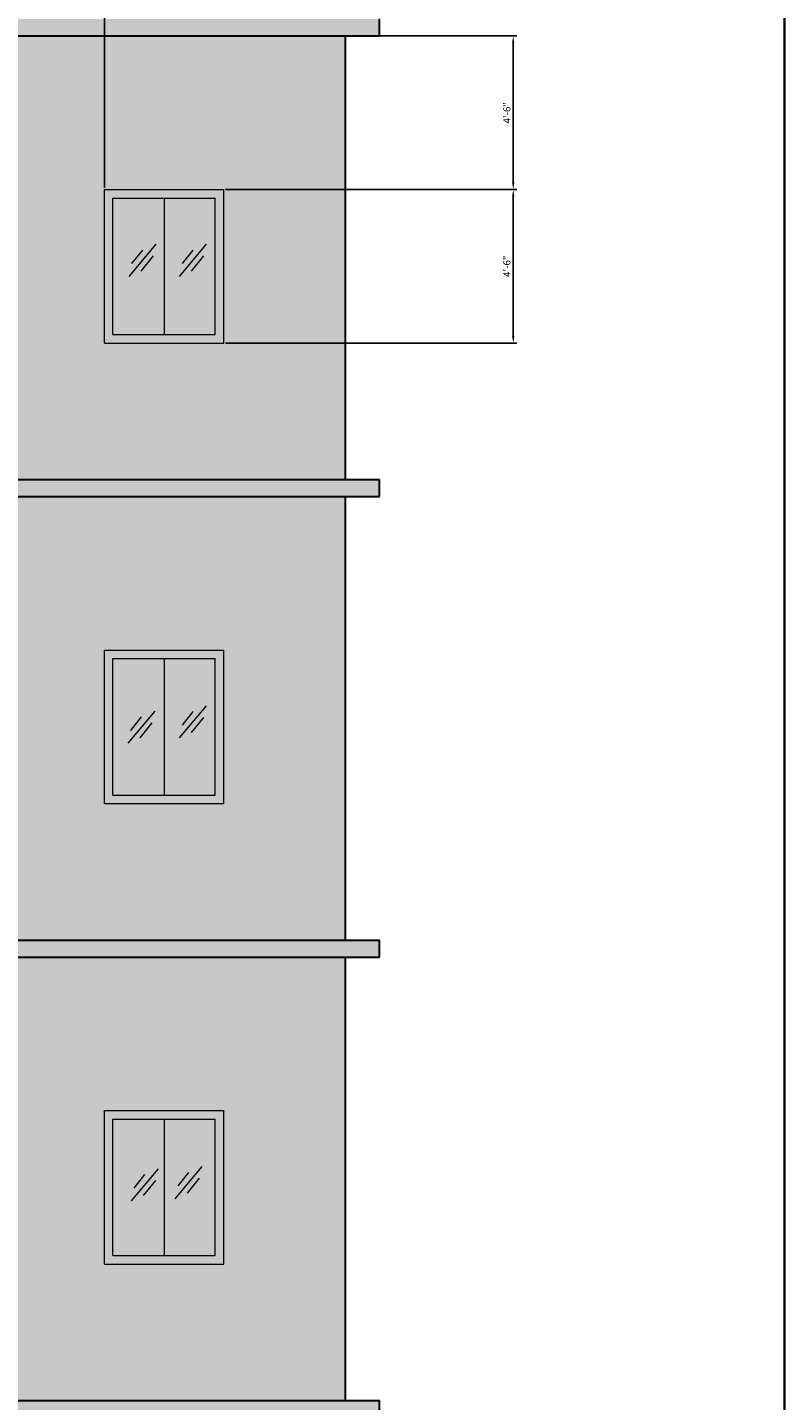
# Model space of a CAD drawing. Units: inches. Extents: x 2391 to 16591, y 7259 to 10239.
# Tile 15 of 27: x 3888 to 4154, y 7746 to 8229. Entities that reach past the tile are written whole.
import ezdxf

# ---------------------------------------------------------------- set-up
doc = ezdxf.new("R2010")
doc.units = ezdxf.units.IN
for name, color, linetype, lineweight in [('A-ANNO-DIMS', 4, 'Continuous', 18), ('A-ANNO-TTLB', 7, 'Continuous', 35), ('A-ELEV', 7, 'Continuous', 30), ('A-ELEV-GLAZ', 4, 'Continuous', 18), ('A-ELEV-GLAZ-PATT', 141, 'Continuous', 13), ('A-ELEV-PATT', 8, 'Continuous', 13), ('A-ELEV-SURF-PATT', 253, 'Continuous', 13)]:
    doc.layers.add(name, color=color, linetype=linetype, lineweight=lineweight)
doc.styles.get("Standard").update_dxf_attribs({"font": 'arial.ttf'})
doc.dimstyles.new('ISO-25', dxfattribs={"dimtxt": 2.5, "dimasz": 2.5, "dimexe": 1.25, "dimexo": 0.625, "dimtad": 1, "dimdec": 0, "dimlunit": 3, "dimtxsty": 'Standard', "dimcen": 2.5, "dimadec": 0, "dimazin": 0, "dimtfac": 1, "dimtdec": 0, "dimtmove": 0, "dimatfit": 3, "dimfxl": 1, "dimarcsym": 0})

# ---------------------------------------------------------------- blocks, each defined once
blk = doc.blocks.new('GLASS-REFLECTION-WINDOW')
for p, q in [((0, 0), (9.5, 11.3)), ((1, 4.52), (4.76, 9.26)), ((4.26, 1.91), (8.52, 7.21))]:
    blk.add_line(p, q)
blk = doc.blocks.new('*D95')
at = {"layer": 'A-ANNO-DIMS', "color": 0, "lineweight": -2, "transparency": 16777216}
for p, q in [((3802.21, 8172.81), (3802.21, 8381.48)), ((3804.71, 8380.23), (3912.46, 8380.23)), ((3914.96, 8172.81), (3914.96, 8381.48))]:
    blk.add_line(p, q, dxfattribs=at)
at = {"layer": 'A-ANNO-DIMS', "color": 0, "transparency": 16777216}
for points in [[(3804.71, 8380.65), (3804.71, 8379.81), (3802.21, 8380.23)], [(3912.46, 8380.65), (3912.46, 8379.81), (3914.96, 8380.23)]]:
    blk.add_solid(points, dxfattribs=at)
at = {"layer": 'Defpoints', "color": 0, "transparency": 16777216}
for p in [(3914.96, 8380.23), (3802.21, 8172.18), (3914.96, 8172.18)]:
    blk.add_point(p, dxfattribs=at)
at = {"layer": 'A-ANNO-DIMS', "color": 0, "transparency": 16777216, "insert": (3858.58, 8382.13), "char_height": 2.5, "attachment_point": 5}
blk.add_mtext('9\'-5"', dxfattribs=at)
blk = doc.blocks.new('*D96')
at = {"layer": 'A-ANNO-DIMS', "color": 0, "lineweight": -2, "transparency": 16777216}
for p, q in [((4000.33, 8226.18), (4060.01, 8226.18)), ((4058.76, 8223.68), (4058.76, 8174.68)), ((3957.58, 8172.18), (4060.01, 8172.18))]:
    blk.add_line(p, q, dxfattribs=at)
at = {"layer": 'A-ANNO-DIMS', "color": 0, "transparency": 16777216}
for points in [[(4058.34, 8223.68), (4059.18, 8223.68), (4058.76, 8226.18)], [(4058.34, 8174.68), (4059.18, 8174.68), (4058.76, 8172.18)]]:
    blk.add_solid(points, dxfattribs=at)
at = {"layer": 'Defpoints', "color": 0, "transparency": 16777216}
for p in [(3999.71, 8226.18), (3956.96, 8172.18), (4058.76, 8172.18)]:
    blk.add_point(p, dxfattribs=at)
at = {"layer": 'A-ANNO-DIMS', "color": 0, "transparency": 16777216, "insert": (4056.86, 8199.18), "char_height": 2.5, "attachment_point": 5, "rotation": 90}
blk.add_mtext('4\'-6"', dxfattribs=at)
blk = doc.blocks.new('*D97')
at = {"layer": 'A-ANNO-DIMS', "color": 0, "lineweight": -2, "transparency": 16777216}
for p, q in [((3957.58, 8172.18), (4060.01, 8172.18)), ((4058.76, 8169.68), (4058.76, 8120.68)), ((3957.58, 8118.18), (4060.01, 8118.18))]:
    blk.add_line(p, q, dxfattribs=at)
at = {"layer": 'A-ANNO-DIMS', "color": 0, "transparency": 16777216}
for points in [[(4058.34, 8169.68), (4059.18, 8169.68), (4058.76, 8172.18)], [(4058.34, 8120.68), (4059.18, 8120.68), (4058.76, 8118.18)]]:
    blk.add_solid(points, dxfattribs=at)
at = {"layer": 'Defpoints', "color": 0, "transparency": 16777216}
for p in [(3956.96, 8172.18), (3956.96, 8118.18), (4058.76, 8118.18)]:
    blk.add_point(p, dxfattribs=at)
at = {"layer": 'A-ANNO-DIMS', "color": 0, "transparency": 16777216, "insert": (4056.86, 8145.18), "char_height": 2.5, "attachment_point": 5, "rotation": 90}
blk.add_mtext('4\'-6"', dxfattribs=at)

msp = doc.modelspace()

# ---------------------------------------------------------------- hatches: boundary and pattern name
at = {"layer": 'A-ELEV-GLAZ-PATT'}
h = msp.add_hatch(color=256, dxfattribs=at)
h.dxf.hatch_style = 1
h.paths.add_polyline_path([(3750.21, 8172.18), (3720.21, 8172.18), (3720.21, 8154.18), (3750.21, 8154.18)])
h.paths.add_polyline_path([(3747.21, 8169.18), (3747.21, 8157.18), (3723.21, 8157.18), (3723.21, 8169.18)], flags=16)
h.paths.add_polyline_path([(3802.21, 8172.18), (3802.21, 8118.18), (3844.21, 8118.18), (3844.21, 8172.18)])
h.paths.add_polyline_path([(3841.21, 8169.18), (3841.21, 8121.18), (3805.21, 8121.18), (3805.21, 8169.18)], flags=16)
h.paths.add_polyline_path([(3956.96, 8172.18), (3914.96, 8172.18), (3914.96, 8118.18), (3956.96, 8118.18)])
h.paths.add_polyline_path([(3953.96, 8169.18), (3953.96, 8121.18), (3917.96, 8121.18), (3917.96, 8169.18)], flags=16)
h.paths.add_polyline_path([(3720.21, 8010.18), (3720.21, 7992.18), (3750.21, 7992.18), (3750.21, 8010.18)])
h.paths.add_polyline_path([(3747.21, 8007.18), (3747.21, 7995.18), (3723.21, 7995.18), (3723.21, 8007.18)], flags=16)
h.paths.add_polyline_path([(3802.21, 8010.18), (3802.21, 7956.18), (3844.21, 7956.18), (3844.21, 8010.18)])
h.paths.add_polyline_path([(3841.21, 8007.18), (3841.21, 7959.18), (3805.21, 7959.18), (3805.21, 8007.18)], flags=16)
h.paths.add_polyline_path([(3914.96, 8010.18), (3914.96, 7956.18), (3956.96, 7956.18), (3956.96, 8010.18)])
h.paths.add_polyline_path([(3917.96, 8007.18), (3953.96, 8007.18), (3953.96, 7959.18), (3917.96, 7959.18)], flags=16)
h.paths.add_polyline_path([(3750.21, 7848.18), (3720.21, 7848.18), (3720.21, 7830.18), (3750.21, 7830.18)])
h.paths.add_polyline_path([(3747.21, 7845.18), (3747.21, 7833.18), (3723.21, 7833.18), (3723.21, 7845.18)], flags=16)
h.paths.add_polyline_path([(3844.21, 7848.18), (3802.21, 7848.18), (3802.21, 7794.18), (3844.21, 7794.18)])
h.paths.add_polyline_path([(3805.21, 7845.18), (3841.21, 7845.18), (3841.21, 7797.18), (3805.21, 7797.18)], flags=16)
h.paths.add_polyline_path([(3914.96, 7848.18), (3914.96, 7794.18), (3956.96, 7794.18), (3956.96, 7848.18)])
h.paths.add_polyline_path([(3917.96, 7845.18), (3953.96, 7845.18), (3953.96, 7797.18), (3917.96, 7797.18)], flags=16)
h = msp.add_hatch(color=256, dxfattribs=at)
h.dxf.hatch_style = 1
h.paths.add_polyline_path([(3735.21, 8169.18), (3723.21, 8169.18), (3723.21, 8157.18), (3735.21, 8157.18)])
h.paths.add_polyline_path([(3747.21, 8169.18), (3735.21, 8169.18), (3735.21, 8157.18), (3747.21, 8157.18)])
h.paths.add_polyline_path([(3823.21, 8169.18), (3805.21, 8169.18), (3805.21, 8121.18), (3823.21, 8121.18)])
h.paths.add_polyline_path([(3841.21, 8169.18), (3823.21, 8169.18), (3823.21, 8121.18), (3841.21, 8121.18)])
h.paths.add_polyline_path([(3935.96, 8169.18), (3917.96, 8169.18), (3917.96, 8121.18), (3935.96, 8121.18)])
h.paths.add_polyline_path([(3953.96, 8169.18), (3935.96, 8169.18), (3935.96, 8121.18), (3953.96, 8121.18)])
h.paths.add_polyline_path([(3735.21, 8007.18), (3723.21, 8007.18), (3723.21, 7995.18), (3735.21, 7995.18)])
h.paths.add_polyline_path([(3747.21, 8007.18), (3735.21, 8007.18), (3735.21, 7995.18), (3747.21, 7995.18)])
h.paths.add_polyline_path([(3823.21, 8007.18), (3805.21, 8007.18), (3805.21, 7959.18), (3823.21, 7959.18)])
h.paths.add_polyline_path([(3841.21, 8007.18), (3823.21, 8007.18), (3823.21, 7959.18), (3841.21, 7959.18)])
h.paths.add_polyline_path([(3935.96, 8007.18), (3917.96, 8007.18), (3917.96, 7959.18), (3935.96, 7959.18)])
h.paths.add_polyline_path([(3953.96, 8007.18), (3935.96, 8007.18), (3935.96, 7959.18), (3953.96, 7959.18)])
h.paths.add_polyline_path([(3735.21, 7845.18), (3723.21, 7845.18), (3723.21, 7833.18), (3735.21, 7833.18)])
h.paths.add_polyline_path([(3747.21, 7845.18), (3735.21, 7845.18), (3735.21, 7833.18), (3747.21, 7833.18)])
h.paths.add_polyline_path([(3823.21, 7845.18), (3805.21, 7845.18), (3805.21, 7797.18), (3823.21, 7797.18)])
h.paths.add_polyline_path([(3841.21, 7845.18), (3823.21, 7845.18), (3823.21, 7797.18), (3841.21, 7797.18)])
h.paths.add_polyline_path([(3935.96, 7845.18), (3917.96, 7845.18), (3917.96, 7797.18), (3935.96, 7797.18)])
h.paths.add_polyline_path([(3953.96, 7845.18), (3935.96, 7845.18), (3935.96, 7797.18), (3953.96, 7797.18)])
at = {"layer": 'A-ELEV-PATT'}
h = msp.add_hatch(dxfattribs=at)
h.set_pattern_fill('BRSTONE', color=256)
h.paths.add_polyline_path([(3999.71, 8226.18), (3881.21, 8226.18), (3881.21, 8070.18), (3999.71, 8070.18)])
h.paths.add_polyline_path([(3956.96, 8118.18), (3914.96, 8118.18), (3914.96, 8172.18), (3956.96, 8172.18)], flags=16)
h.paths.add_polyline_path([(3953.96, 8121.18), (3917.96, 8121.18), (3917.96, 8169.18), (3953.96, 8169.18)], flags=0)
h.paths.add_polyline_path([(3999.71, 8064.18), (3881.21, 8064.18), (3881.21, 7908.18), (3999.71, 7908.18)])
h.paths.add_polyline_path([(3956.96, 7956.18), (3914.96, 7956.18), (3914.96, 8010.18), (3956.96, 8010.18)], flags=16)
h.paths.add_polyline_path([(3953.96, 7959.18), (3917.96, 7959.18), (3917.96, 8007.18), (3953.96, 8007.18)], flags=0)
h.paths.add_polyline_path([(3999.71, 7902.18), (3881.21, 7902.18), (3881.21, 7746.18), (3999.71, 7746.18)])
h.paths.add_polyline_path([(3956.96, 7794.18), (3914.96, 7794.18), (3914.96, 7848.18), (3956.96, 7848.18)], flags=16)
h.paths.add_polyline_path([(3953.96, 7797.18), (3917.96, 7797.18), (3917.96, 7845.18), (3953.96, 7845.18)], flags=0)
h.paths.add_polyline_path([(3999.71, 7740.18), (3567.71, 7740.18), (3567.71, 7697.18), (3760.71, 7697.18), (3760.71, 7706.18), (3755.71, 7706.18), (3755.71, 7711.18), (3774.71, 7711.18), (3774.71, 7706.18), (3769.71, 7706.18), (3769.71, 7677.02), (3772.21, 7677.02), (3772.21, 7679.02), (3774.71, 7679.02), (3774.71, 7704.18), (3843.71, 7704.18), (3843.71, 7589.18), (3774.71, 7589.18), (3774.71, 7584.18), (3913.71, 7584.18), (3913.71, 7589.18), (3844.71, 7589.18), (3844.71, 7704.18), (3913.71, 7704.18), (3913.71, 7679.02), (3916.21, 7679.02), (3916.21, 7677.02), (3918.71, 7677.02), (3918.71, 7706.18), (3913.71, 7706.18), (3913.71, 7711.18), (3932.71, 7711.18), (3932.71, 7706.18), (3927.71, 7706.18), (3927.71, 7697.18), (3999.71, 7697.18)])
h.paths.add_polyline_path([(3918.71, 7675.02), (3916.21, 7675.02), (3916.21, 7673.02), (3913.71, 7673.02), (3913.71, 7618.89), (3916.21, 7618.89), (3916.21, 7616.89), (3918.71, 7616.89)], flags=17)
h.paths.add_polyline_path([(3918.71, 7614.89), (3916.21, 7614.89), (3916.21, 7612.89), (3913.71, 7612.89), (3913.71, 7584.18), (3918.71, 7584.18)], flags=17)
h.paths.add_polyline_path([(3774.71, 7673.02), (3772.21, 7673.02), (3772.21, 7675.02), (3769.71, 7675.02), (3769.71, 7616.89), (3772.21, 7616.89), (3772.21, 7618.89), (3774.71, 7618.89)], flags=17)
h.paths.add_polyline_path([(3774.71, 7612.89), (3772.21, 7612.89), (3772.21, 7614.89), (3769.71, 7614.89), (3769.71, 7584.18), (3774.71, 7584.18), (3774.71, 7589.18)], flags=17)
at = {"layer": 'A-ELEV-SURF-PATT'}
h = msp.add_hatch(color=256, dxfattribs=at)
h.dxf.hatch_style = 1
h.paths.add_polyline_path([(4011.71, 7740.18), (4011.71, 7746.18), (3555.71, 7746.18), (3555.71, 7740.18)])
h.paths.add_polyline_path([(4011.71, 7902.18), (4011.71, 7908.18), (3555.71, 7908.18), (3555.71, 7902.18)])
h.paths.add_polyline_path([(4011.71, 8064.18), (4011.71, 8070.18), (3555.71, 8070.18), (3555.71, 8064.18)])
h.paths.add_polyline_path([(3555.71, 8232.18), (3555.71, 8226.18), (4011.71, 8226.18), (4011.71, 8232.18)])
h.paths.add_polyline_path([(3778.21, 8333.18), (3778.21, 8328.18), (3978.71, 8328.18), (3978.71, 8333.18)])

# ---------------------------------------------------------------- linework, layer by layer
at = {"layer": 'A-ANNO-TTLB'}
msp.add_lwpolyline([(2391.28, 10239.38), (4154.2, 10239.38), (4154.2, 7258.54), (2391.28, 7258.54)], close=True, dxfattribs=at)
at = {"layer": 'A-ELEV'}
for p, q in [((4011.71, 8226.18), (4011.71, 8232.18)), ((3555.71, 8226.18), (4011.71, 8226.18)), ((3999.71, 8070.18), (3999.71, 8226.18)), ((3555.71, 8070.18), (4011.71, 8070.18)), ((4011.71, 8064.18), (4011.71, 8070.18)), ((3555.71, 8064.18), (4011.71, 8064.18)), ((3999.71, 7908.18), (3999.71, 8064.18)), ((3555.71, 7908.18), (4011.71, 7908.18)), ((4011.71, 7902.18), (4011.71, 7908.18)), ((3555.71, 7902.18), (4011.71, 7902.18)), ((3999.71, 7746.18), (3999.71, 7902.18)), ((3555.71, 7746.18), (4011.71, 7746.18)), ((4011.71, 7740.18), (4011.71, 7746.18))]:
    msp.add_line(p, q, dxfattribs=at)
at = {"layer": 'A-ELEV-GLAZ'}
for p, q in [((3914.96, 8172.18), (3956.96, 8172.18)), ((3914.96, 8118.18), (3914.96, 8172.18)), ((3917.96, 8169.18), (3953.96, 8169.18)), ((3917.96, 8121.18), (3917.96, 8169.18)), ((3935.96, 8169.18), (3935.96, 8121.18)), ((3953.96, 8121.18), (3953.96, 8169.18)), ((3956.96, 8118.18), (3956.96, 8172.18)), ((3917.96, 8121.18), (3953.96, 8121.18)), ((3914.96, 8118.18), (3956.96, 8118.18)), ((3914.96, 8010.18), (3956.96, 8010.18)), ((3914.96, 7956.18), (3914.96, 8010.18)), ((3956.96, 7956.18), (3956.96, 8010.18)), ((3917.96, 8007.18), (3953.96, 8007.18)), ((3917.96, 7959.18), (3917.96, 8007.18)), ((3935.96, 8007.18), (3935.96, 7959.18)), ((3953.96, 7959.18), (3953.96, 8007.18)), ((3914.96, 7956.18), (3956.96, 7956.18)), ((3917.96, 7959.18), (3953.96, 7959.18)), ((3914.96, 7848.18), (3956.96, 7848.18)), ((3914.96, 7794.18), (3914.96, 7848.18)), ((3917.96, 7845.18), (3953.96, 7845.18)), ((3917.96, 7797.18), (3917.96, 7845.18)), ((3935.96, 7845.18), (3935.96, 7797.18)), ((3953.96, 7797.18), (3953.96, 7845.18)), ((3956.96, 7794.18), (3956.96, 7848.18)), ((3917.96, 7797.18), (3953.96, 7797.18)), ((3914.96, 7794.18), (3956.96, 7794.18))]:
    msp.add_line(p, q, dxfattribs=at)

# ---------------------------------------------------------------- block references
for p in [(3923.65, 8141.6), (3941.37, 8141.6), (3941.37, 7979.28), (3923.26, 7977.37), (3924.46, 7816.38), (3939.88, 7817.17)]:
    msp.add_blockref('GLASS-REFLECTION-WINDOW', p, dxfattribs=at)

# ---------------------------------------------------------------- dimensions: what is measured, and where the dimension line sits
at = {"layer": 'A-ANNO-DIMS'}
dim = msp.add_linear_dim(base=(3914.959246, 8380.230453), p1=(3802.209246, 8172.180453), p2=(3914.959246, 8172.180453), dimstyle='ISO-25', override={"dimdec": 1, "dimlfac": 1, "dimrnd": 0, "dimzin": 1, "dimdsep": 46, "dimlunit": 4, "dimfrac": 2}, dxfattribs=at)
dim.commit()
dim.dimension.update_dxf_attribs({"geometry": '*D95', "text_midpoint": (3858.584246, 8382.13188547)})
for base, p1, p2, picture, middle in [((4058.76, 8172.18), (3999.71, 8226.18), (3956.96, 8172.18), '*D96', (4056.86, 8199.18)), ((4058.76, 8118.18), (3956.96, 8172.18), (3956.96, 8118.18), '*D97', (4056.86, 8145.18))]:
    dim = msp.add_linear_dim(base=base, p1=p1, p2=p2, angle=90, dimstyle='ISO-25', override={"dimdec": 1, "dimlfac": 1, "dimrnd": 0, "dimzin": 1, "dimdsep": 46, "dimlunit": 4, "dimfrac": 2}, dxfattribs=at)
    dim.commit()
    dim.dimension.update_dxf_attribs({"geometry": picture, "text_midpoint": middle})

doc.saveas('drawing.dxf')
